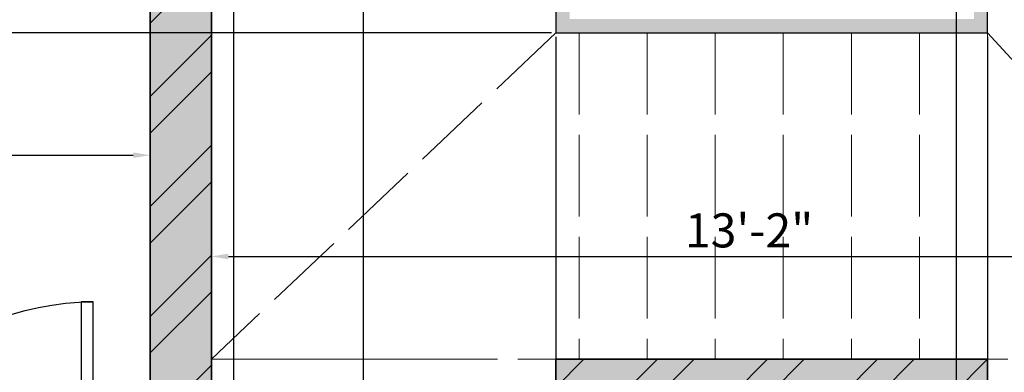
# Model space of a CAD drawing. Units: inches. Extents: x 1804 to 3296, y 909 to 2477.
# Tile 7 of 31: x 2130 to 2275, y 1174 to 1226. Entities that reach past the tile are written whole.
import ezdxf

# ---------------------------------------------------------------- set-up
doc = ezdxf.new("R2010")
doc.units = ezdxf.units.IN
doc.linetypes.add('ACAD_ISO02W100', pattern=[15, 12, -3])
for name, color, linetype, lineweight in [('A-ANNO-DIMS', 2, 'Continuous', 18), ('A-ANNO-TTLB', 156, 'Continuous', 35), ('A-FLOR-PATT', 8, 'Continuous', 13), ('A-FLOR-STRS', 7, 'Continuous', 25), ('A-FLOR-STRS-OVHD', 8, 'ACAD_ISO02W100', 18), ('A-GLAZ-OVHD', 130, 'ACAD_ISO02W100', 18), ('A-WALL-PATT', 10, 'Continuous', 13), ('DOOR', 30, 'Continuous', 25), ('WALL', 10, 'Continuous', 35), ('WIND', 130, 'Continuous', 18)]:
    doc.layers.add(name, color=color, linetype=linetype, lineweight=lineweight)
doc.styles.get("Standard").update_dxf_attribs({"font": 'arial.ttf'})
doc.dimstyles.new('ISO-25', dxfattribs={"dimtxt": 5, "dimasz": 2.5, "dimexe": 1.25, "dimexo": 0.625, "dimtad": 1, "dimdec": 0, "dimlunit": 4, "dimtxsty": 'Standard', "dimcen": 2.5, "dimadec": 0, "dimazin": 0, "dimtfac": 1, "dimtdec": 0, "dimtmove": 0, "dimatfit": 3, "dimfxl": 1, "dimarcsym": 0})

# ---------------------------------------------------------------- blocks, each defined once
blk = doc.blocks.new('*U2')
for p, q in [((0, 0), (0, -6)), ((40, 0), (40, -6))]:
    blk.add_line(p, q)
blk.add_lwpolyline([(0, 0), (0, 40), (1.75, 40), (1.75, 0)], close=True)
blk.add_arc((0, 0), 40, 0, 90)
blk = doc.blocks.new('*D19')
at = {"layer": 'A-ANNO-DIMS', "color": 0, "lineweight": -2, "transparency": 16777216}
for p, q in [((2158.58, 1176.26), (2158.58, 1192)), ((2316.54, 1176.26), (2316.54, 1192)), ((2161.08, 1190.75), (2314.04, 1190.75))]:
    blk.add_line(p, q, dxfattribs=at)
at = {"layer": 'A-ANNO-DIMS', "color": 0, "lineweight": 100, "transparency": 16777216}
for points in [[(2161.08, 1191.16), (2161.08, 1190.33), (2158.58, 1190.75)], [(2314.04, 1191.16), (2314.04, 1190.33), (2316.54, 1190.75)]]:
    blk.add_solid(points, dxfattribs=at)
at = {"layer": 'Defpoints', "color": 0, "lineweight": 100, "transparency": 16777216}
for p in [(2316.54, 1190.75), (2158.58, 1175.63), (2316.54, 1175.63)]:
    blk.add_point(p, dxfattribs=at)
at = {"layer": 'A-ANNO-DIMS', "color": 0, "transparency": 16777216, "insert": (2237.56, 1193.93), "char_height": 5, "attachment_point": 5}
blk.add_mtext('13\'-2"', dxfattribs=at)
blk = doc.blocks.new('*D22')
at = {"layer": 'A-ANNO-DIMS', "color": 0, "lineweight": -2, "transparency": 16777216}
for p, q in [((1934.58, 1147.69), (1934.58, 1206.88)), ((2149.58, 1147.69), (2149.58, 1206.88)), ((1937.08, 1205.63), (2147.08, 1205.63))]:
    blk.add_line(p, q, dxfattribs=at)
at = {"layer": 'A-ANNO-DIMS', "color": 0, "lineweight": 100, "transparency": 16777216}
for points in [[(1937.08, 1206.05), (1937.08, 1205.22), (1934.58, 1205.63)], [(2147.08, 1206.05), (2147.08, 1205.22), (2149.58, 1205.63)]]:
    blk.add_solid(points, dxfattribs=at)
at = {"layer": 'Defpoints', "color": 0, "lineweight": 100, "transparency": 16777216}
for p in [(2149.58, 1205.63), (1934.58, 1147.07), (2149.58, 1147.07)]:
    blk.add_point(p, dxfattribs=at)
at = {"layer": 'A-ANNO-DIMS', "color": 0, "transparency": 16777216, "insert": (2042.08, 1208.77), "char_height": 5, "attachment_point": 5}
blk.add_mtext('17\'-11"', dxfattribs=at)
blk = doc.blocks.new('*D56')
at = {"layer": 'A-ANNO-DIMS', "color": 0, "lineweight": -2, "transparency": 16777216}
for p, q in [((2180.87, 1680.42), (2180.87, 975.89)), ((2268, 1680.42), (2268, 975.89)), ((2183.37, 977.14), (2265.5, 977.14))]:
    blk.add_line(p, q, dxfattribs=at)
at = {"layer": 'A-ANNO-DIMS', "color": 0, "lineweight": 100, "transparency": 16777216}
for points in [[(2183.37, 977.56), (2183.37, 976.72), (2180.87, 977.14)], [(2265.5, 977.56), (2265.5, 976.72), (2268, 977.14)]]:
    blk.add_solid(points, dxfattribs=at)
at = {"layer": 'Defpoints', "color": 0, "lineweight": 100, "transparency": 16777216}
for p in [(2180.87, 1681.04), (2268, 1681.04), (2268, 977.14)]:
    blk.add_point(p, dxfattribs=at)
at = {"layer": 'A-ANNO-DIMS', "color": 0, "transparency": 16777216, "insert": (2224.44, 980.32), "char_height": 5, "attachment_point": 5}
blk.add_mtext('7\'-3"', dxfattribs=at)
blk = doc.blocks.new('*D59')
at = {"layer": 'A-ANNO-DIMS', "color": 0, "lineweight": -2, "transparency": 16777216}
for p, q in [((2121.83, 1590.3), (2121.83, 975.89)), ((2161.83, 1590.3), (2161.83, 975.89)), ((2124.33, 977.14), (2159.33, 977.14))]:
    blk.add_line(p, q, dxfattribs=at)
at = {"layer": 'A-ANNO-DIMS', "color": 0, "lineweight": 100, "transparency": 16777216}
for points in [[(2124.33, 977.56), (2124.33, 976.72), (2121.83, 977.14)], [(2159.33, 977.56), (2159.33, 976.72), (2161.83, 977.14)]]:
    blk.add_solid(points, dxfattribs=at)
at = {"layer": 'Defpoints', "color": 0, "lineweight": 100, "transparency": 16777216}
for p in [(2121.83, 1590.92), (2161.83, 1590.92), (2161.83, 977.14)]:
    blk.add_point(p, dxfattribs=at)
at = {"layer": 'A-ANNO-DIMS', "color": 0, "transparency": 16777216, "insert": (2141.83, 980.32), "char_height": 5, "attachment_point": 5}
blk.add_mtext('3\'-4"', dxfattribs=at)
blk = doc.blocks.new('*D69')
at = {"layer": 'A-ANNO-DIMS', "color": 0, "lineweight": -2, "transparency": 16777216}
for p, q in [((2209.19, 1223.01), (2209.19, 975.89)), ((2272.59, 1223.01), (2272.59, 975.89)), ((2211.69, 977.14), (2270.09, 977.14))]:
    blk.add_line(p, q, dxfattribs=at)
at = {"layer": 'A-ANNO-DIMS', "color": 0, "lineweight": 100, "transparency": 16777216}
for points in [[(2211.69, 977.56), (2211.69, 976.72), (2209.19, 977.14)], [(2270.09, 977.56), (2270.09, 976.72), (2272.59, 977.14)]]:
    blk.add_solid(points, dxfattribs=at)
at = {"layer": 'Defpoints', "color": 0, "lineweight": 100, "transparency": 16777216}
for p in [(2209.19, 1223.63), (2272.59, 1223.63), (2272.59, 977.14)]:
    blk.add_point(p, dxfattribs=at)
at = {"layer": 'A-ANNO-DIMS', "color": 0, "transparency": 16777216, "insert": (2240.89, 980.35), "char_height": 5, "attachment_point": 5}
blk.add_mtext('5\'-3 1/2"', dxfattribs=at)
blk = doc.blocks.new('*D70')
at = {"layer": 'A-ANNO-DIMS', "color": 0, "lineweight": -2, "transparency": 16777216}
for p, q in [((2208.56, 1271.63), (1880.63, 1271.63)), ((1881.88, 1226.13), (1881.88, 1269.13)), ((2208.56, 1223.63), (1880.63, 1223.63))]:
    blk.add_line(p, q, dxfattribs=at)
at = {"layer": 'A-ANNO-DIMS', "color": 0, "lineweight": 100, "transparency": 16777216}
for points in [[(1881.47, 1269.13), (1882.3, 1269.13), (1881.88, 1271.63)], [(1881.47, 1226.13), (1882.3, 1226.13), (1881.88, 1223.63)]]:
    blk.add_solid(points, dxfattribs=at)
at = {"layer": 'Defpoints', "color": 0, "lineweight": 100, "transparency": 16777216}
for p in [(1881.88, 1271.63), (2209.19, 1271.63), (2209.19, 1223.63)]:
    blk.add_point(p, dxfattribs=at)
at = {"layer": 'A-ANNO-DIMS', "color": 0, "transparency": 16777216, "insert": (1878.7, 1247.63), "char_height": 5, "attachment_point": 5, "rotation": 90}
blk.add_mtext('4\'-0"', dxfattribs=at)

msp = doc.modelspace()

# ---------------------------------------------------------------- hatches: boundary and pattern name
at = {"layer": 'A-ANNO-TTLB'}
h = msp.add_hatch(color=256, dxfattribs=at)
h.dxf.hatch_style = 1
h.paths.add_polyline_path([(3294.53, 2476.54), (1803.79, 2476.54), (1805.43, 909.47), (3296.17, 909.47)])
h.paths.add_polyline_path([(1811, 914.33), (1812.79, 2467.54), (3285.53, 2467.54), (3283.74, 914.33)], flags=16)
h.paths.add_polyline_path([(1925.58, 1062.77), (1925.58, 1138.07), (1925.58, 1539.88), (1925.58, 1793.38), (1925.58, 1830.04), (2325.54, 1830.04), (2325.54, 1793.38), (2325.54, 1586.42), (2325.54, 1138.07), (2325.54, 1062.77)], flags=0)
h.paths.add_polyline_path([(1997.22, 1029.4), (2008.85, 1037.96), (2008.85, 1020.84)], flags=0)
h.paths.add_polyline_path([(1934.58, 1138.07), (1934.58, 1147.07), (2078.77, 1147.07), (2078.77, 1138.07), (2060.94, 1138.07)], flags=0)
h.paths.add_polyline_path([(1944.35, 1138.07), (1944.35, 1147.07), (2056.05, 1147.07), (2056.05, 1138.07)], flags=0)
h.paths.add_polyline_path([(2222.24, 1037.96), (2233.87, 1029.4), (2222.24, 1020.84)], flags=0)
h.paths.add_polyline_path([(2061.94, 1139.07), (2061.94, 1146.07), (2077.77, 1146.07), (2077.77, 1139.07)], flags=0)
h.paths.add_polyline_path([(2149.58, 1138.07), (2149.58, 1269.44), (2158.58, 1269.44), (2158.58, 1326.69), (2149.58, 1326.69), (2149.58, 1340.94), (2139.6, 1340.94), (2139.6, 1434.25), (2149.58, 1434.25), (2149.58, 1447.36), (2158.58, 1447.36), (2158.58, 1423.87), (2158.58, 1408.06), (2198.46, 1408.06), (2198.46, 1412.56), (2282.65, 1412.56), (2282.65, 1465.94), (2316.54, 1465.94), (2316.54, 1590.92), (2192.86, 1590.92), (2192.86, 1595.3), (2291.17, 1595.3), (2291.17, 1590.92), (2316.54, 1590.92), (2316.54, 1784.38), (2300.24, 1784.38), (2300.24, 1757.47), (2268, 1757.47), (2268, 1681.04), (2180.87, 1681.04), (2180.87, 1757.47), (2148.63, 1757.47), (2148.63, 1784.38), (2119.08, 1784.38), (2119.08, 1585.58), (2114.58, 1585.58), (2114.58, 1784.38), (2064.11, 1784.38), (2046.28, 1784.38), (2046.28, 1760.38), (1958.58, 1760.38), (1958.58, 1664.38), (1934.58, 1664.38), (1934.58, 1784.38), (1934.58, 1793.38), (2046.28, 1793.38), (2064.11, 1793.38), (2119.08, 1793.38), (2230.78, 1793.38), (2230.78, 1784.38), (2268, 1784.38), (2300.24, 1784.38), (2316.54, 1784.38), (2316.54, 1590.92), (2316.54, 1373.73), (2316.54, 1138.07)], flags=0)
h.paths.add_polyline_path([(2209.19, 1166.63), (2209.19, 1175.63), (2158.58, 1175.63), (2209.19, 1223.63), (2209.19, 1231.63), (2183.88, 1231.63), (2183.88, 1301.66), (2242.59, 1301.66), (2242.59, 1326.69), (2316.54, 1326.69), (2272.59, 1271.63), (2272.59, 1223.63), (2316.54, 1175.63), (2272.59, 1175.63), (2272.59, 1166.63)], flags=0)
h.paths.add_polyline_path([(1947.77, 1345.22), (1947.77, 1457.48), (1991.2, 1457.48), (1991.2, 1451.7), (1991.2, 1352.18), (1991.2, 1345.22)], flags=0)
h.paths.add_polyline_path([(2209.19, 1271.63), (2262.59, 1271.63), (2262.59, 1311.85), (2272.59, 1301.66), (2272.59, 1271.63), (2269.92, 1269.63), (2270.59, 1269.63), (2270.59, 1225.63), (2211.19, 1225.63), (2211.19, 1269.63), (2211.86, 1269.63)], flags=0)
h.paths.add_polyline_path([(2000.34, 1378.21), (2000.34, 1429.71), (2025.22, 1429.71), (2025.22, 1378.21)], flags=0)
h.paths.add_polyline_path([(2001.34, 1379.21), (2001.34, 1428.71), (2024.22, 1428.71), (2024.22, 1379.21)], flags=0)
h.paths.add_polyline_path([(2012.34, 1390.21), (2012.34, 1417.71), (2013.22, 1417.71), (2013.22, 1390.21)], flags=0)
h.paths.add_polyline_path([(2237.56, 1331.19), (2237.56, 1340.18), (2238.62, 1340.18), (2238.62, 1386.84), (2241.04, 1386.84), (2242.06, 1386.84), (2242.06, 1408.06), (2316.54, 1331.19)], flags=0)
h.paths.add_polyline_path([(1953.73, 1464.35), (1953.73, 1498.59), (1981.74, 1498.59), (1981.74, 1464.35)], flags=0)
h.paths.add_polyline_path([(1987.63, 1462.08), (1987.63, 1500.95), (2104.07, 1500.95), (2104.07, 1462.08), (2099.27, 1462.08), (1993.6, 1462.08)], flags=0)
h.paths.add_polyline_path([(1956.06, 1481.47, -1), (1979.41, 1481.47, -1)], flags=0)
edge = h.paths.add_edge_path(flags=0)
edge.add_ellipse((2299.53, 1438.37), major_axis=(0.31, 21.36), ratio=0.670333, start_angle=0, end_angle=360)
h.paths.add_polyline_path([(2297.39, 1438.37, -1), (2301.67, 1438.37, -1)], flags=0)
h.paths.add_polyline_path([(2591.54, 1163.23), (2591.54, 1179.38), (2591.54, 1379.68), (2591.54, 1395.84), (2734.5, 1395.84), (2734.5, 1379.68), (2734.5, 1179.38), (2734.5, 1163.23)], flags=0)
h.paths.add_polyline_path([(2592.54, 1164.23), (2592.54, 1166.23), (2733.5, 1166.23), (2733.5, 1164.23)], flags=0)
h.paths.add_polyline_path([(2592.54, 1180.38), (2592.54, 1378.68), (2733.5, 1378.68), (2733.5, 1180.38)], flags=0)
h.paths.add_polyline_path([(2593.54, 1181.38), (2593.54, 1377.68), (2732.5, 1377.68), (2732.5, 1181.38)], flags=0)
h.paths.add_polyline_path([(2594.54, 1182.38), (2594.54, 1376.68), (2731.5, 1376.68), (2731.5, 1182.38)], flags=0)
h.paths.add_polyline_path([(1936.95, 1697.46), (1936.95, 1736.46), (1955.41, 1736.46), (1955.41, 1697.46)], flags=0)
h.paths.add_polyline_path([(1938.48, 1718.36), (1938.48, 1734.92), (1953.65, 1734.92), (1953.65, 1718.36)], flags=0)
h.paths.add_polyline_path([(1944.75, 1726.64, -1), (1947.37, 1726.64, -1)], flags=0)
h.paths.add_polyline_path([(2592.54, 1394.84), (2733.5, 1394.84), (2733.5, 1392.84), (2592.54, 1392.84)], flags=0)
h.paths.add_polyline_path([(1976.61, 1762.5), (1976.61, 1781.44), (2012.79, 1781.44), (2012.79, 1762.5)], flags=0)
h.paths.add_polyline_path([(1979.57, 1771.97, -1), (1991.39, 1771.97, -1)], flags=0)
h.paths.add_polyline_path([(1995.36, 1771.97, -1), (2007.18, 1771.97, -1)], flags=0)
h.paths.add_polyline_path([(2251.51, 1744.53), (2268, 1730.05), (2251.51, 1730.05)], flags=0)
h.paths.add_polyline_path([(2047.28, 1785.38), (2047.28, 1792.38), (2063.11, 1792.38), (2063.11, 1785.38)], flags=0)
h.paths.add_polyline_path([(2155.08, 1770.92, -1), (2174.42, 1770.92, -1)], flags=0)
h.paths.add_polyline_path([(2188.59, 1758.27), (2188.59, 1772.81), (2222.3, 1772.81), (2222.3, 1758.27)], flags=0)
h.paths.add_polyline_path([(2223.97, 1758.27), (2223.97, 1772.81), (2257.68, 1772.81), (2257.68, 1758.27)], flags=0)
h.paths.add_polyline_path([(2274.45, 1770.92, -1), (2293.8, 1770.92, -1)], flags=0)
h.paths.add_polyline_path([(2591.54, 1582.09), (2591.54, 1782.39), (2734.5, 1782.39), (2734.5, 1582.09)], flags=0)
h.paths.add_polyline_path([(2592.54, 1583.09), (2592.54, 1781.39), (2733.5, 1781.39), (2733.5, 1583.09)], flags=0)
h.paths.add_polyline_path([(2593.54, 1584.09), (2593.54, 1780.39), (2732.5, 1780.39), (2732.5, 1584.09)], flags=0)
h.paths.add_polyline_path([(2594.54, 1585.09), (2594.54, 1779.39), (2731.5, 1779.39), (2731.5, 1585.09)], flags=0)
h.paths.add_polyline_path([(1922.17, 1978.79), (1922.17, 2295.08), (1922.17, 2296.08), (2115.67, 2296.08), (2115.67, 2384.31), (2115.67, 2385.31), (2322.12, 2385.31), (2323.12, 2385.31), (2323.12, 1979.79), (2323.12, 1978.79), (1923.17, 1978.79)], flags=0)
h.paths.add_polyline_path([(1922.17, 1978.79), (1922.17, 2051.31), (1922.17, 2214.86), (1922.17, 2296.08), (2115.67, 2296.08), (2115.67, 2385.31), (2323.12, 2385.31), (2323.12, 2280.42), (2323.12, 1978.79), (2115.67, 1978.79)], flags=0)
h.paths.add_polyline_path([(1923.17, 1979.79), (1923.17, 2050.31), (2115.67, 2050.31), (2115.67, 2051.31), (1923.17, 2051.31), (1923.17, 2213.86), (1923.17, 2214.86), (1923.17, 2295.08), (1990.02, 2295.08), (1990.02, 2214.86), (1991.02, 2214.86), (1991.02, 2295.08), (2115.67, 2295.08), (2115.67, 1979.79), (2116.67, 1979.79), (2116.67, 2304.18), (2116.67, 2384.31), (2322.12, 2384.31), (2322.12, 2280.42), (2322.12, 1979.79), (2115.67, 1979.79)], flags=0)
h.paths.add_polyline_path([(2972.46, 1192.5), (2972.46, 1196.92), (2995.47, 1196.92), (2995.47, 1255.47), (2995.09, 1255.47), (2987.42, 1249.39), (2980.08, 1255.47), (2978.05, 1255.47), (2978.05, 1257.24), (2995.47, 1257.24), (2995.47, 1261.58), (3015.37, 1261.58), (3015.37, 1333.28), (3015.37, 1414.4), (3032.82, 1414.4), (3032.82, 1333.28), (3032.82, 1261.58), (3052.66, 1261.58), (3052.66, 1255.47), (3079.86, 1255.47), (3078.72, 1254.57), (3081.47, 1252.29), (3078.56, 1249.99), (3075.81, 1252.26), (3072.57, 1249.69), (3070.36, 1251.52), (3067.67, 1249.39), (3060.34, 1255.47), (3052.66, 1255.47), (3052.66, 1196.92), (3054.58, 1196.92), (3074, 1196.92), (3074, 1192.5), (3052.66, 1192.5), (2995.47, 1192.5)], flags=0)
h.paths.add_polyline_path([(2490.75, 1979.27), (2490.75, 1980.27), (2596.87, 1980.27), (2596.87, 2051.8), (2596.87, 2052.8), (2596.87, 2216.35), (2596.87, 2297.57), (2717.32, 2297.57), (2710.57, 2305.62), (2724.07, 2305.62), (2717.32, 2297.57), (2782.37, 2297.57), (2782.37, 2395.8), (3006.82, 2395.8), (3006.82, 1981.27), (3093.73, 1981.27), (3093.73, 1980.27), (3047.51, 1980.27), (3046.37, 1979.37), (3049.11, 1977.1), (3046.2, 1974.79), (3043.46, 1977.07), (3040.21, 1974.49), (3038, 1976.32), (3035.32, 1974.2), (3027.98, 1980.27), (2871.83, 1980.27), (2871.83, 1981.27), (2791.37, 1981.27), (2791.37, 2050.8), (2597.87, 2050.8), (2597.87, 1980.27), (2597.87, 1979.27), (2546.27, 1979.27), (2545.12, 1978.37), (2547.87, 1976.1), (2544.96, 1973.79), (2542.22, 1976.07), (2538.97, 1973.49), (2536.76, 1975.32), (2534.07, 1973.2), (2526.74, 1979.27)], flags=0)
h.paths.add_polyline_path([(2597.87, 2051.8), (2606.87, 2051.8), (2606.87, 2258.39), (2597.87, 2258.39), (2597.87, 2296.57), (2606.87, 2296.57), (2606.87, 2262.39), (2782.37, 2262.39), (2782.37, 2296.57), (2790.37, 2296.57), (2790.37, 2262.39), (2791.37, 2262.39), (2791.37, 2305.67), (2791.37, 2385.8), (2996.82, 2385.8), (2996.82, 2339.85), (3006.82, 2339.85), (3006.82, 2250.12), (2997.82, 2250.12), (2997.82, 1981.27), (2996.82, 1981.27), (2872.83, 1981.27), (2872.83, 1991.8), (2871.83, 1991.8), (2871.83, 2050.8), (2790.37, 2050.8), (2597.87, 2050.8)], flags=0)
h.paths.add_polyline_path([(2179.93, 2153.92), (2179.93, 2353.97), (2259.98, 2353.97), (2259.98, 2153.92)], flags=0)
h.paths.add_polyline_path([(2180.93, 2154.92), (2180.93, 2352.97), (2258.98, 2352.97), (2258.98, 2154.92)], flags=0)
h.paths.add_polyline_path([(2960.87, 1608.49), (2960.87, 1753.62), (3070.9, 1753.62), (3070.9, 1608.49)], flags=0)
h.paths.add_polyline_path([(2961.87, 1609.49), (2961.87, 1752.62), (3069.9, 1752.62), (3069.9, 1609.49)], flags=0)
h.paths.add_polyline_path([(2962.87, 1610.49), (2962.87, 1751.62), (3068.9, 1751.62), (3068.9, 1610.49)], flags=0)
h.paths.add_polyline_path([(2963.87, 1611.49), (2963.87, 1750.62), (3067.9, 1750.62), (3067.9, 1611.49)], flags=0)
h.paths.add_polyline_path([(2782.37, 2051.8), (2782.37, 2216.32), (2791.37, 2216.32), (2791.37, 2051.8), (2872.83, 2051.8), (2872.83, 2068.56), (2884.67, 2068.56), (2884.67, 2085.33), (2896.51, 2085.33), (2896.51, 2102.09), (2908.36, 2102.09), (2908.36, 2118.85), (2920.2, 2118.85), (2920.2, 2135.62), (2932.05, 2135.62), (2932.05, 2145.3), (2925.08, 2145.3), (2925.08, 2203.2), (2996.82, 2203.2), (2996.82, 2145.3), (2953.82, 2145.3), (2872.83, 2051.8), (2790.37, 2051.8)], flags=0)
h.paths.add_polyline_path([(2717.32, 2238.65), (2710.57, 2246.7), (2724.07, 2246.7)], flags=0)
h.paths.add_polyline_path([(2003.09, 1122.79), (2017.16, 1122.79), (2017.16, 1138.74), (2003.09, 1138.74)], flags=8)
h.paths.add_polyline_path([(2174.76, 1792.72), (2188.83, 1792.72), (2188.83, 1808.66), (2174.76, 1808.66)], flags=8)
h.paths.add_polyline_path([(1987.95, 1792.51), (2002.02, 1792.51), (2002.02, 1808.45), (1987.95, 1808.45)], flags=8)
h.paths.add_polyline_path([(2148.79, 1289.26), (2160.46, 1289.26), (2160.46, 1305.2), (2148.79, 1305.2)], flags=8)
h.paths.add_polyline_path([(2115.36, 1133.57), (2127.04, 1133.57), (2127.04, 1149.51), (2115.36, 1149.51)], flags=8)
h.paths.add_polyline_path([(2237.58, 1421.48), (2249.25, 1421.48), (2249.25, 1437.43), (2237.58, 1437.43)], flags=8)
h.paths.add_polyline_path([(2134.99, 1584.32), (2146.66, 1584.32), (2146.66, 1600.26), (2134.99, 1600.26)], flags=8)
h.paths.add_polyline_path([(2101.95, 1557.31), (2113.62, 1557.31), (2113.62, 1573.25), (2101.95, 1573.25)], flags=8)
h.paths.add_polyline_path([(2937.85, 1156.77), (3120.41, 1156.77), (3120.41, 1185.72), (2937.85, 1185.72)], flags=8)
h.paths.add_polyline_path([(2980.71, 1786.71), (3050.06, 1786.71), (3050.06, 1802.66), (2980.71, 1802.66)], flags=8)
h.paths.add_polyline_path([(2869.28, 1661.96), (2938.62, 1661.96), (2938.62, 1690.8), (2869.28, 1690.8)], flags=8)
h.paths.add_polyline_path([(3092.27, 1674.86), (3161.62, 1674.86), (3161.62, 1690.8), (3092.27, 1690.8)], flags=8)
h.paths.add_polyline_path([(2980.71, 1674.86), (3050.06, 1674.86), (3050.06, 1690.8), (2980.71, 1690.8)], flags=8)
h.paths.add_polyline_path([(2649.07, 1678.23), (2674.53, 1678.23), (2674.53, 1714.76), (2649.07, 1714.76)], flags=8)
h.paths.add_polyline_path([(2530.84, 1981.63), (2549.13, 1981.63), (2549.13, 1997.57), (2530.84, 1997.57)], flags=8)
h.paths.add_polyline_path([(3031.29, 1981.77), (3049.58, 1981.77), (3049.58, 1997.71), (3031.29, 1997.71)], flags=8)
h.paths.add_polyline_path([(2715.38, 1911.9), (2851.54, 1911.9), (2851.54, 1940.85), (2715.38, 1940.85)], flags=8)
h.paths.add_polyline_path([(2015.23, 1927.36), (2205.42, 1927.36), (2205.42, 1956.3), (2015.23, 1956.3)], flags=8)
h.paths.add_polyline_path([(2671.84, 2057.84), (2702.75, 2057.84), (2702.75, 2073.79), (2671.84, 2073.79)], flags=8)
h.paths.add_polyline_path([(2678.5, 2316.52), (2765.26, 2316.52), (2765.26, 2332.46), (2678.5, 2332.46)], flags=8)
h.paths.add_polyline_path([(2678.48, 2271.96), (2736.41, 2271.96), (2736.41, 2287.9), (2678.48, 2287.9)], flags=8)
h.paths.add_polyline_path([(2019.2, 972.79), (2243.21, 972.79), (2243.21, 1001.74), (2019.2, 1001.74)], flags=8)
h.paths.add_polyline_path([(2097.06, 1021.56), (2132.16, 1021.56), (2132.16, 1037.51), (2097.06, 1037.51)], flags=8)
h.paths.add_polyline_path([(2182.47, 1360.48), (2207.35, 1360.48), (2207.35, 1376.42), (2182.47, 1376.42)], flags=8)
h.paths.add_polyline_path([(2261.12, 1361.77), (2295.01, 1361.77), (2295.01, 1377.71), (2261.12, 1377.71)], flags=8)
h.paths.add_polyline_path([(2245.75, 1511.51), (2278.44, 1511.51), (2278.44, 1527.46), (2245.75, 1527.46)], flags=8)
h.paths.add_polyline_path([(1991.16, 1296.29), (2060.51, 1296.29), (2060.51, 1312.23), (1991.16, 1312.23)], flags=8)
h.paths.add_polyline_path([(2187, 1651.35), (2246.71, 1651.35), (2246.71, 1667.29), (2187, 1667.29)], flags=8)
h.paths.add_polyline_path([(1976.49, 1684.81), (2068.63, 1684.81), (2068.63, 1700.76), (1976.49, 1700.76)], flags=8)
at = {"layer": 'A-FLOR-PATT'}
h = msp.add_hatch(color=256, dxfattribs=at)
h.dxf.hatch_style = 1
h.paths.add_polyline_path([(2272.59, 1271.63), (2209.19, 1271.63), (2211.86, 1269.63), (2269.92, 1269.63)], flags=17)
h.paths.add_polyline_path([(2211.19, 1269.63), (2211.86, 1269.63), (2209.19, 1271.63), (2209.19, 1223.63), (2272.59, 1223.63), (2272.59, 1271.63), (2269.92, 1269.63), (2270.59, 1269.63), (2270.59, 1225.63), (2211.19, 1225.63)])
at = {"layer": 'A-WALL-PATT'}
h = msp.add_hatch(color=256, dxfattribs=at)
h.dxf.hatch_style = 1
h.paths.add_polyline_path([(2149.58, 1147.07), (2141.21, 1147.07), (2141.21, 1144.07), (2141.21, 1138.07), (2149.58, 1138.07)])
h.paths.add_polyline_path([(2101.21, 1144.07, -0.01877), (2101.32, 1147.07), (2078.77, 1147.07), (2078.77, 1138.07), (2101.21, 1138.07)])
h.paths.add_polyline_path([(2060.94, 1147.07), (2056.05, 1147.07), (2056.05, 1138.07), (2060.94, 1138.07)])
h.paths.add_polyline_path([(1944.35, 1147.07), (1934.58, 1147.07), (1934.58, 1138.07), (1944.35, 1138.07)])
h.paths.add_polyline_path([(2158.58, 1269.44), (2149.58, 1269.44), (2149.58, 1138.07), (2158.58, 1138.07)])
h.paths.add_polyline_path([(2003.09, 1122.79), (2017.16, 1122.79), (2017.16, 1138.74), (2003.09, 1138.74)], flags=9)
h.paths.add_polyline_path([(2174.76, 1792.72), (2188.83, 1792.72), (2188.83, 1808.66), (2174.76, 1808.66)], flags=9)
h.paths.add_polyline_path([(1987.95, 1792.51), (2002.02, 1792.51), (2002.02, 1808.45), (1987.95, 1808.45)], flags=9)
h.paths.add_polyline_path([(2148.79, 1289.26), (2160.46, 1289.26), (2160.46, 1305.2), (2148.79, 1305.2)], flags=9)
h.paths.add_polyline_path([(2115.36, 1133.57), (2127.04, 1133.57), (2127.04, 1149.51), (2115.36, 1149.51)], flags=9)
h.paths.add_polyline_path([(2237.58, 1421.48), (2249.25, 1421.48), (2249.25, 1437.43), (2237.58, 1437.43)], flags=9)
h.paths.add_polyline_path([(2134.99, 1584.32), (2146.66, 1584.32), (2146.66, 1600.26), (2134.99, 1600.26)], flags=9)
h.paths.add_polyline_path([(2101.95, 1557.31), (2113.62, 1557.31), (2113.62, 1573.25), (2101.95, 1573.25)], flags=9)
h.paths.add_polyline_path([(2937.85, 1156.77), (3120.41, 1156.77), (3120.41, 1185.72), (2937.85, 1185.72)], flags=9)
h.paths.add_polyline_path([(2980.71, 1786.71), (3050.06, 1786.71), (3050.06, 1802.66), (2980.71, 1802.66)], flags=9)
h.paths.add_polyline_path([(2869.28, 1661.96), (2938.62, 1661.96), (2938.62, 1690.8), (2869.28, 1690.8)], flags=9)
h.paths.add_polyline_path([(3092.27, 1674.86), (3161.62, 1674.86), (3161.62, 1690.8), (3092.27, 1690.8)], flags=9)
h.paths.add_polyline_path([(2980.71, 1674.86), (3050.06, 1674.86), (3050.06, 1690.8), (2980.71, 1690.8)], flags=9)
h.paths.add_polyline_path([(2649.07, 1678.23), (2674.53, 1678.23), (2674.53, 1714.76), (2649.07, 1714.76)], flags=9)
h.paths.add_polyline_path([(2530.84, 1981.63), (2549.13, 1981.63), (2549.13, 1997.57), (2530.84, 1997.57)], flags=9)
h.paths.add_polyline_path([(3031.29, 1981.77), (3049.58, 1981.77), (3049.58, 1997.71), (3031.29, 1997.71)], flags=9)
h.paths.add_polyline_path([(2715.38, 1911.9), (2851.54, 1911.9), (2851.54, 1940.85), (2715.38, 1940.85)], flags=9)
h.paths.add_polyline_path([(2015.23, 1927.36), (2205.42, 1927.36), (2205.42, 1956.3), (2015.23, 1956.3)], flags=9)
h.paths.add_polyline_path([(2671.84, 2057.84), (2702.75, 2057.84), (2702.75, 2073.79), (2671.84, 2073.79)], flags=9)
h.paths.add_polyline_path([(2678.5, 2316.52), (2765.26, 2316.52), (2765.26, 2332.46), (2678.5, 2332.46)], flags=9)
h.paths.add_polyline_path([(2678.48, 2271.96), (2736.41, 2271.96), (2736.41, 2287.9), (2678.48, 2287.9)], flags=9)
h.paths.add_polyline_path([(2019.2, 972.79), (2243.21, 972.79), (2243.21, 1001.74), (2019.2, 1001.74)], flags=9)
h.paths.add_polyline_path([(2097.06, 1021.56), (2132.16, 1021.56), (2132.16, 1037.51), (2097.06, 1037.51)], flags=9)
h.paths.add_polyline_path([(2182.47, 1360.48), (2207.35, 1360.48), (2207.35, 1376.42), (2182.47, 1376.42)], flags=9)
h.paths.add_polyline_path([(2261.12, 1361.77), (2295.01, 1361.77), (2295.01, 1377.71), (2261.12, 1377.71)], flags=9)
h.paths.add_polyline_path([(2245.75, 1511.51), (2278.44, 1511.51), (2278.44, 1527.46), (2245.75, 1527.46)], flags=9)
h.paths.add_polyline_path([(1991.16, 1296.29), (2060.51, 1296.29), (2060.51, 1312.23), (1991.16, 1312.23)], flags=9)
h.paths.add_polyline_path([(2187, 1651.35), (2246.71, 1651.35), (2246.71, 1667.29), (2187, 1667.29)], flags=9)
h.paths.add_polyline_path([(1976.49, 1684.81), (2068.63, 1684.81), (2068.63, 1700.76), (1976.49, 1700.76)], flags=9)
h = msp.add_hatch(color=256, dxfattribs=at)
h.dxf.hatch_style = 1
h.paths.add_polyline_path([(2158.58, 1275.49), (2155.29, 1275.49), (2149.58, 1275.49), (2149.58, 1269.44), (2158.58, 1269.44)])
h.paths.add_polyline_path([(2158.58, 1326.69), (2149.58, 1326.69), (2149.58, 1319.33), (2155.29, 1319.33), (2158.58, 1319.33)])
h.paths.add_polyline_path([(2158.58, 1402.2), (2158.58, 1423.87), (2158.58, 1447.36), (2149.58, 1447.36), (2149.58, 1423.87), (2149.58, 1340.94), (2149.58, 1326.69), (2158.58, 1326.69), (2158.58, 1354.23)])
h.paths.add_polyline_path([(1965.87, 1658.79), (1965.87, 1679.09), (1955.57, 1679.09), (1955.57, 1658.79)], flags=9)
h.paths.add_polyline_path([(2293.18, 1677.29), (2293.18, 1697.58), (2282.88, 1697.58), (2282.88, 1677.29)], flags=9)
h.paths.add_polyline_path([(2271.13, 1545.23), (2287.53, 1545.23), (2287.53, 1555.53), (2271.13, 1555.53)], flags=9)
h.paths.add_polyline_path([(2303.26, 1488.52), (2303.26, 1508.82), (2292.95, 1508.82), (2292.95, 1488.52)], flags=9)
h.paths.add_polyline_path([(2271.13, 1393.15), (2287.53, 1393.15), (2287.53, 1403.45), (2271.13, 1403.45)], flags=9)
h.paths.add_polyline_path([(2306.48, 1361.45), (2306.48, 1377.86), (2296.18, 1377.86), (2296.18, 1361.45)], flags=9)
h.paths.add_polyline_path([(2189.9, 1340.62), (2206.31, 1340.62), (2206.31, 1350.92), (2189.9, 1350.92)], flags=9)
h.paths.add_polyline_path([(2174.54, 1361.45), (2174.54, 1377.86), (2164.23, 1377.86), (2164.23, 1361.45)], flags=9)
h.paths.add_polyline_path([(2304.24, 1240.8), (2304.24, 1261.09), (2293.94, 1261.09), (2293.94, 1240.8)], flags=9)
h.paths.add_polyline_path([(2227.19, 1188.73), (2247.49, 1188.73), (2247.49, 1199.03), (2227.19, 1199.03)], flags=9)
h.paths.add_polyline_path([(2181.93, 1144.21), (2181.93, 1160.62), (2171.63, 1160.62), (2171.63, 1144.21)], flags=9)
h.paths.add_polyline_path([(1968.21, 1333.34), (1968.21, 1353.64), (1957.91, 1353.64), (1957.91, 1333.34)], flags=9)
h.paths.add_polyline_path([(2029.78, 1203.53), (2053.95, 1203.53), (2053.95, 1213.83), (2029.78, 1213.83)], flags=9)
h.paths.add_polyline_path([(2576.51, 1671.88), (2576.51, 1692.17), (2566.21, 1692.17), (2566.21, 1671.88)], flags=9)
h.paths.add_polyline_path([(2566.99, 1269.67), (2566.99, 1289.96), (2556.68, 1289.96), (2556.68, 1269.67)], flags=9)
h.paths.add_polyline_path([(2581.85, 1269.17), (2581.85, 1289.46), (2571.54, 1289.46), (2571.54, 1269.17)], flags=9)
h.paths.add_polyline_path([(2650.71, 1409.75), (2674.89, 1409.75), (2674.89, 1420.05), (2650.71, 1420.05)], flags=9)
h.paths.add_polyline_path([(2003.09, 1122.79), (2017.16, 1122.79), (2017.16, 1138.74), (2003.09, 1138.74)], flags=9)
h.paths.add_polyline_path([(2174.76, 1792.72), (2188.83, 1792.72), (2188.83, 1808.66), (2174.76, 1808.66)], flags=9)
h.paths.add_polyline_path([(1987.95, 1792.51), (2002.02, 1792.51), (2002.02, 1808.45), (1987.95, 1808.45)], flags=9)
h.paths.add_polyline_path([(2148.79, 1289.26), (2160.46, 1289.26), (2160.46, 1305.2), (2148.79, 1305.2)], flags=9)
h.paths.add_polyline_path([(2115.36, 1133.57), (2127.04, 1133.57), (2127.04, 1149.51), (2115.36, 1149.51)], flags=9)
h.paths.add_polyline_path([(2237.58, 1421.48), (2249.25, 1421.48), (2249.25, 1437.43), (2237.58, 1437.43)], flags=9)
h.paths.add_polyline_path([(2134.99, 1584.32), (2146.66, 1584.32), (2146.66, 1600.26), (2134.99, 1600.26)], flags=9)
h.paths.add_polyline_path([(2101.95, 1557.31), (2113.62, 1557.31), (2113.62, 1573.25), (2101.95, 1573.25)], flags=9)
h.paths.add_polyline_path([(2937.85, 1156.77), (3120.41, 1156.77), (3120.41, 1185.72), (2937.85, 1185.72)], flags=9)
h.paths.add_polyline_path([(2980.71, 1786.71), (3050.06, 1786.71), (3050.06, 1802.66), (2980.71, 1802.66)], flags=9)
h.paths.add_polyline_path([(2869.28, 1661.96), (2938.62, 1661.96), (2938.62, 1690.8), (2869.28, 1690.8)], flags=9)
h.paths.add_polyline_path([(3092.27, 1674.86), (3161.62, 1674.86), (3161.62, 1690.8), (3092.27, 1690.8)], flags=9)
h.paths.add_polyline_path([(2980.71, 1674.86), (3050.06, 1674.86), (3050.06, 1690.8), (2980.71, 1690.8)], flags=9)
h.paths.add_polyline_path([(2649.07, 1678.23), (2674.53, 1678.23), (2674.53, 1714.76), (2649.07, 1714.76)], flags=9)
h.paths.add_polyline_path([(2530.84, 1981.63), (2549.13, 1981.63), (2549.13, 1997.57), (2530.84, 1997.57)], flags=9)
h.paths.add_polyline_path([(3031.29, 1981.77), (3049.58, 1981.77), (3049.58, 1997.71), (3031.29, 1997.71)], flags=9)
h.paths.add_polyline_path([(2715.38, 1911.9), (2851.54, 1911.9), (2851.54, 1940.85), (2715.38, 1940.85)], flags=9)
h.paths.add_polyline_path([(2015.23, 1927.36), (2205.42, 1927.36), (2205.42, 1956.3), (2015.23, 1956.3)], flags=9)
h.paths.add_polyline_path([(2671.84, 2057.84), (2702.75, 2057.84), (2702.75, 2073.79), (2671.84, 2073.79)], flags=9)
h.paths.add_polyline_path([(2678.5, 2316.52), (2765.26, 2316.52), (2765.26, 2332.46), (2678.5, 2332.46)], flags=9)
h.paths.add_polyline_path([(2678.48, 2271.96), (2736.41, 2271.96), (2736.41, 2287.9), (2678.48, 2287.9)], flags=9)
h.paths.add_polyline_path([(2019.2, 972.79), (2243.21, 972.79), (2243.21, 1001.74), (2019.2, 1001.74)], flags=9)
h.paths.add_polyline_path([(2097.06, 1021.56), (2132.16, 1021.56), (2132.16, 1037.51), (2097.06, 1037.51)], flags=9)
h.paths.add_polyline_path([(2182.47, 1360.48), (2207.35, 1360.48), (2207.35, 1376.42), (2182.47, 1376.42)], flags=9)
h.paths.add_polyline_path([(2261.12, 1361.77), (2295.01, 1361.77), (2295.01, 1377.71), (2261.12, 1377.71)], flags=9)
h.paths.add_polyline_path([(2245.75, 1511.51), (2278.44, 1511.51), (2278.44, 1527.46), (2245.75, 1527.46)], flags=9)
h.paths.add_polyline_path([(1991.16, 1296.29), (2060.51, 1296.29), (2060.51, 1312.23), (1991.16, 1312.23)], flags=9)
h.paths.add_polyline_path([(2187, 1651.35), (2246.71, 1651.35), (2246.71, 1667.29), (2187, 1667.29)], flags=9)
h.paths.add_polyline_path([(1976.49, 1684.81), (2068.63, 1684.81), (2068.63, 1700.76), (1976.49, 1700.76)], flags=9)
h = msp.add_hatch(dxfattribs=at)
h.set_pattern_fill('ANSI32', color=256, scale=1.2)
h.set_pattern_definition([(45, (0, 196.207), (-8.08223, 8.08223), []), (45, (5.388, 196.207), (-8.08223, 8.08223), [])])
h.paths.add_polyline_path([(1934.58, 1784.38), (1934.58, 1793.38), (1925.58, 1793.38), (1925.58, 1539.88), (2119.08, 1539.88), (2119.08, 1545.58), (2114.58, 1545.58), (2114.58, 1544.38), (1934.58, 1544.38)])
h.paths.add_polyline_path([(2114.58, 1793.38), (2064.11, 1793.38), (2064.11, 1784.38), (2114.58, 1784.38)], flags=17)
h.paths.add_polyline_path([(2325.54, 1793.38), (2230.78, 1793.38), (2230.78, 1784.38), (2268, 1784.38), (2300.24, 1784.38), (2316.54, 1784.38), (2316.54, 1590.92), (2316.54, 1586.42), (2325.54, 1586.42)])
h.paths.add_polyline_path([(1944.35, 1147.07), (1934.58, 1147.07), (1934.58, 1138.07), (1944.35, 1138.07)])
h.paths.add_polyline_path([(2101.21, 1144.07, -0.01877), (2101.32, 1147.07), (2078.77, 1147.07), (2078.77, 1138.07), (2101.21, 1138.07)])
h.paths.add_polyline_path([(1934.58, 1539.88), (1925.58, 1539.88), (1925.58, 1138.07), (1934.58, 1138.07), (1934.58, 1147.07)])
h.paths.add_polyline_path([(2325.54, 1586.42), (2316.54, 1586.42), (2316.54, 1373.73), (2316.54, 1138.07), (2325.54, 1138.07), (2325.54, 1228.97)])
h.paths.add_polyline_path([(2158.58, 1423.87), (2158.58, 1447.36), (2149.58, 1447.36), (2149.58, 1423.87), (2149.58, 1340.94), (2149.58, 1326.69), (2158.58, 1326.69), (2158.58, 1354.23), (2158.58, 1402.2)])
h.paths.add_polyline_path([(2316.54, 1412.56), (2282.65, 1412.56), (2273.09, 1412.56), (2273.09, 1408.06), (2316.54, 1408.06)])
h.paths.add_polyline_path([(2273.09, 1412.56), (2242.06, 1412.56), (2242.06, 1408.06), (2273.09, 1408.06)])
h.paths.add_polyline_path([(2237.56, 1412.56), (2198.46, 1412.56), (2198.46, 1408.06), (2237.56, 1408.06)])
h.paths.add_polyline_path([(2242.06, 1408.06), (2237.56, 1408.06), (2237.56, 1386.84), (2242.06, 1386.84)])
h.paths.add_polyline_path([(2242.06, 1412.56), (2237.56, 1412.56), (2237.56, 1408.06), (2242.06, 1408.06)])
h.paths.add_polyline_path([(2158.58, 1269.44), (2149.58, 1269.44), (2149.58, 1138.07), (2158.58, 1138.07)])
h.paths.add_polyline_path([(2149.58, 1147.07), (2141.21, 1147.07), (2141.21, 1144.07), (2141.21, 1138.07), (2149.58, 1138.07)])
h.paths.add_polyline_path([(2272.59, 1175.63), (2209.19, 1175.63), (2209.19, 1166.63), (2272.59, 1166.63)])
h.paths.add_polyline_path([(2237.56, 1446.21), (2242.06, 1446.21), (2242.06, 1586.42), (2237.56, 1586.42)])
h.paths.add_polyline_path([(2242.06, 1414.58), (2237.56, 1414.58), (2237.56, 1412.56), (2242.06, 1412.56)])
h = msp.add_hatch(color=256, dxfattribs=at)
h.dxf.hatch_style = 1
h.paths.add_polyline_path([(2114.58, 1793.38), (2064.11, 1793.38), (2064.11, 1784.38), (2114.58, 1784.38)])
h.paths.add_polyline_path([(2119.08, 1793.38), (2114.58, 1793.38), (2114.58, 1585.58), (2119.08, 1585.58)])
h.paths.add_polyline_path([(2325.54, 1793.38), (2230.78, 1793.38), (2230.78, 1784.38), (2268, 1784.38), (2316.54, 1784.38), (2316.54, 1590.92), (2316.54, 1586.42), (2325.54, 1586.42)])
h.paths.add_polyline_path([(2316.54, 1331.19), (2158.58, 1331.19), (2158.58, 1326.69), (2316.54, 1326.69)])
h.paths.add_polyline_path([(2242.06, 1408.06), (2237.56, 1408.06), (2237.56, 1386.84), (2242.06, 1386.84)])
h.paths.add_polyline_path([(2242.06, 1412.56), (2237.56, 1412.56), (2237.56, 1408.06), (2242.06, 1408.06)])
h.paths.add_polyline_path([(2237.56, 1412.56), (2198.46, 1412.56), (2198.46, 1408.06), (2237.56, 1408.06)])
h.paths.add_polyline_path([(2273.09, 1412.56), (2242.06, 1412.56), (2242.06, 1408.06), (2273.09, 1408.06)])
h.paths.add_polyline_path([(2316.54, 1412.56), (2282.65, 1412.56), (2273.09, 1412.56), (2273.09, 1408.06), (2316.54, 1408.06)])
h.paths.add_polyline_path([(2325.54, 1586.42), (2316.54, 1586.42), (2316.54, 1373.73), (2316.54, 1138.07), (2325.54, 1138.07), (2325.54, 1228.97)])
h.paths.add_polyline_path([(2272.59, 1175.63), (2209.19, 1175.63), (2209.19, 1166.63), (2272.59, 1166.63)])

# ---------------------------------------------------------------- linework, layer by layer
at = {"layer": 'A-FLOR-STRS'}
for p, q in [((2209.19, 1271.63), (2209.19, 1223.63)), ((2272.59, 1223.63), (2272.59, 1271.63)), ((2209.19, 1223.63), (2272.59, 1223.63))]:
    msp.add_line(p, q, dxfattribs=at)
at = {"layer": 'A-FLOR-STRS-OVHD'}
for p, q in [((2209.19, 1223.63), (2158.58, 1175.63)), ((2212.59, 1223.63), (2212.59, 1175.63)), ((2222.59, 1223.63), (2222.59, 1175.63)), ((2232.59, 1223.63), (2232.59, 1175.63)), ((2242.59, 1223.63), (2242.59, 1175.63)), ((2252.59, 1223.63), (2252.59, 1175.63)), ((2262.59, 1223.63), (2262.59, 1175.63)), ((2272.59, 1223.63), (2272.59, 1175.63)), ((2272.59, 1223.63), (2316.54, 1175.63))]:
    msp.add_line(p, q, dxfattribs=at)
at = {"layer": 'A-GLAZ-OVHD'}
msp.add_line((2158.58, 1175.63), (2316.54, 1175.63), dxfattribs=at)
at = {"layer": 'WALL'}
for p, q in [((2158.58, 1138.07), (2158.58, 1354.23)), ((2149.58, 1138.07), (2149.58, 1269.44))]:
    msp.add_line(p, q, dxfattribs=at)
msp.add_lwpolyline([(2209.19, 1175.63), (2272.59, 1175.63), (2272.59, 1166.63), (2209.19, 1166.63)], close=True, dxfattribs=at)
at = {"layer": 'WIND'}
for p, q in [((2158.58, 1175.63), (2194.58, 1175.63)), ((2194.58, 1175.63), (2200.58, 1175.63))]:
    msp.add_line(p, q, dxfattribs=at)

# ---------------------------------------------------------------- block references
at = {"layer": 'DOOR', "xscale": -1}
msp.add_blockref('*U2', (2141.21, 1144.07), dxfattribs=at)

# ---------------------------------------------------------------- dimensions: what is measured, and where the dimension line sits
at = {"layer": 'A-ANNO-DIMS'}
for base, p1, p2, override, picture, middle in [((2268, 977.14), (2180.87, 1681.04), (2268, 1681.04), {"dimdec": 1, "dimlfac": 1, "dimrnd": 0, "dimzin": 1, "dimdsep": 46, "dimlunit": 4, "dimfrac": 2}, '*D56', (2224.44, 980.32)), ((2161.83, 977.14), (2121.83, 1590.92), (2161.83, 1590.92), {"dimdec": 1, "dimlfac": 1, "dimrnd": 0, "dimzin": 1, "dimdsep": 46, "dimlunit": 4, "dimfrac": 2}, '*D59', (2141.83, 980.32)), ((2272.59, 977.14), (2209.19, 1223.63), (2272.59, 1223.63), {"dimdec": 1, "dimlfac": 1, "dimrnd": 0, "dimzin": 1, "dimdsep": 46, "dimlunit": 4, "dimfrac": 2}, '*D69', (2240.89, 980.35)), ((2149.58, 1205.63), (1934.58, 1147.07), (2149.58, 1147.07), {"dimclrd": 0, "dimclre": 0, "dimclrt": 0}, '*D22', (2042.08, 1208.77)), ((2316.54, 1190.75), (2158.58, 1175.63), (2316.54, 1175.63), {"dimclrd": 0, "dimclre": 0, "dimclrt": 0}, '*D19', (2237.56, 1193.93))]:
    dim = msp.add_linear_dim(base=base, p1=p1, p2=p2, dimstyle='ISO-25', override=override, dxfattribs=at)
    dim.commit()
    dim.dimension.update_dxf_attribs({"geometry": picture, "text_midpoint": middle})
dim = msp.add_linear_dim(base=(1881.88, 1271.63), p1=(2209.19, 1223.63), p2=(2209.19, 1271.63), angle=90, dimstyle='ISO-25', override={"dimdec": 1, "dimlfac": 1, "dimrnd": 0, "dimzin": 1, "dimdsep": 46, "dimlunit": 4, "dimfrac": 2}, dxfattribs=at)
dim.commit()
dim.dimension.update_dxf_attribs({"geometry": '*D70', "text_midpoint": (1878.7, 1247.63)})

doc.saveas('drawing.dxf')
